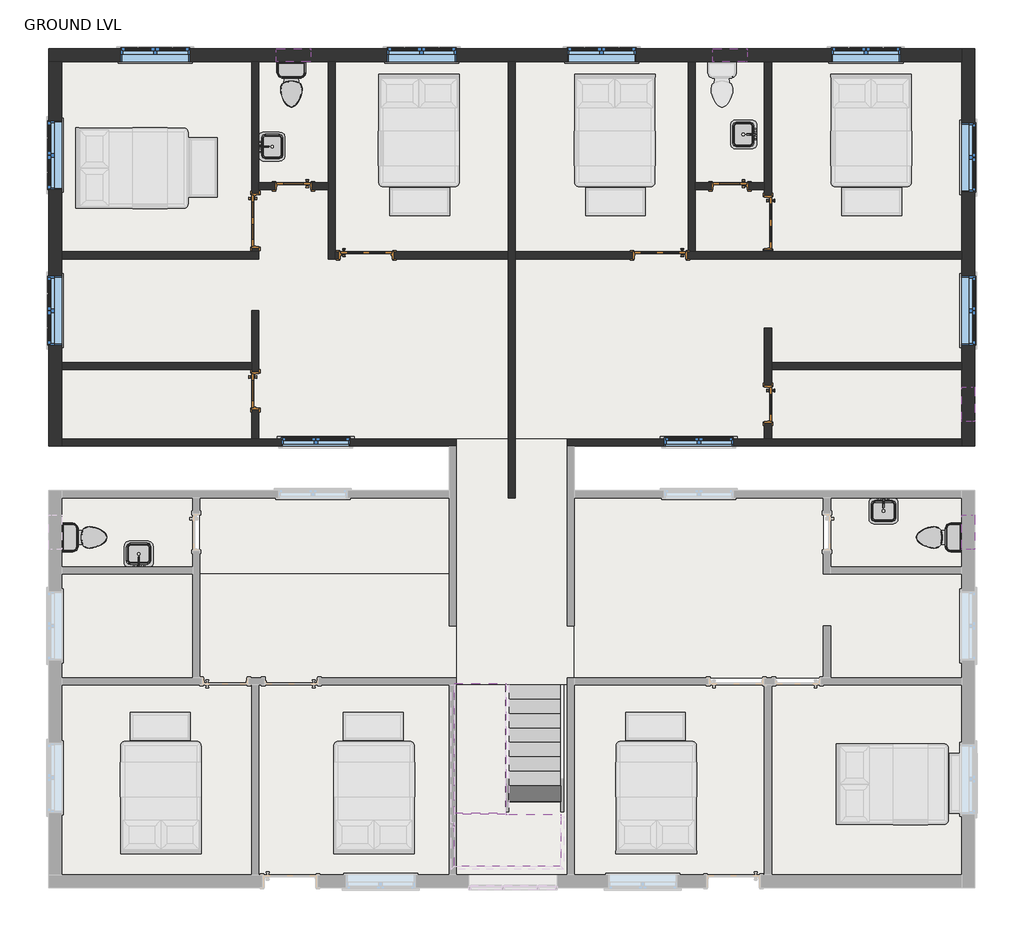
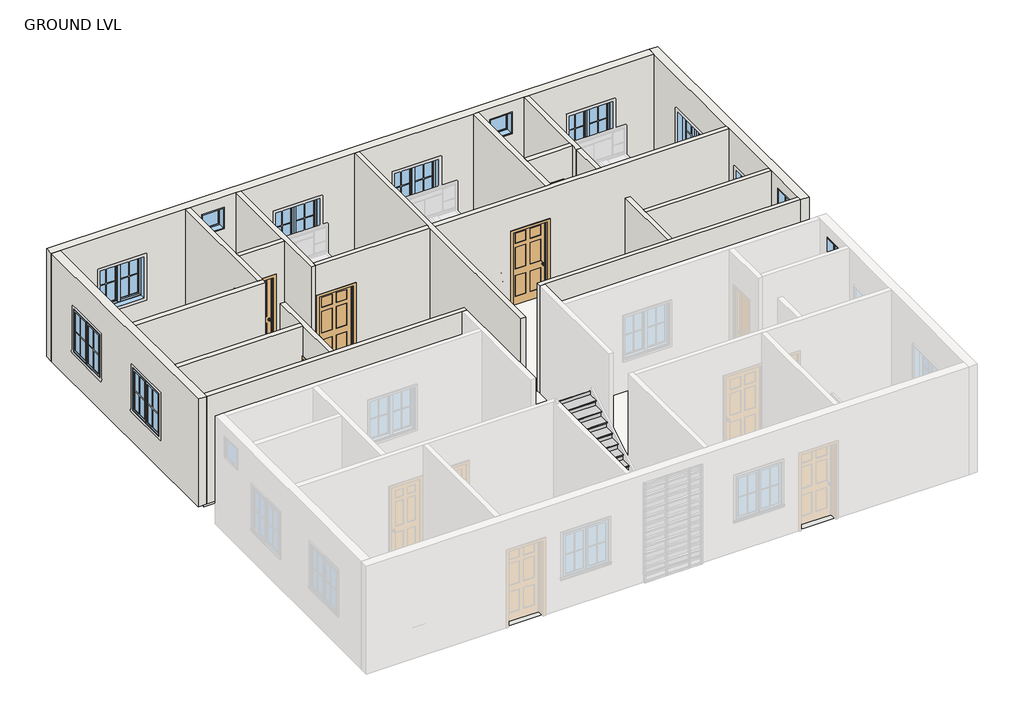
# One storey, part 3 of 4: 20 walls, 14 windows, 8 doors, 7 flow terminals, 7 slabs, 2 stair flights.
"""IFC4 building model written with IfcOpenShell, lengths in millimetres."""

from ifc_helpers import new_model, si_unit, frame, origin, origin_with_axes, place, context, project, spatial, polyline, outline, extrude, faceted_brep, transform, mapped, element, save
from components import door_e337afa5, door_596d7c92, door_c610b25b, door_03e3dfb5, flow_terminal_8d9ea526, toilet_domestic_3d_toilet_domestic_3d_ba6479b0, toilet_domestic_3d_toilet_domestic_3d_30431060, non_monolithic_landing_2d37ff17, stair_flight_38cd46e1, stair_flight_39a519ea, window_80340324, window_9200f5ac, window_c2c97eee

model = new_model("IFC4")

# Units and contexts
model_context = context("Model", 3, world=origin())
ifc_project = project(units=[si_unit("LENGTHUNIT", "METRE", prefix="MILLI")], contexts=[model_context])

# Site, building, storey
site = spatial("IfcSite", under=ifc_project)
building = spatial("IfcBuilding", under=site)
storey = spatial("IfcBuildingStorey", under=building, Name="GROUND LVL", Elevation=0.0)

# Doors
placement = place(None, origin())
door_shape = door_e337afa5(model_context)
element("IfcDoor", 1, ObjectType="Door-Interior-Single-2_Panel-Wood : 24\" x 84\"", at=placement, inside=storey, context=model_context, shape_type="MappedRepresentation", body=[
    mapped(door_shape, transform((-8112.4137331, 4563.2156164, 0.0), x_axis=(-1.0, 0.0, 0.0), y_axis=(0.0, -1.0, 0.0), z_axis=(0.0, 0.0, 1.0))),
])
element("IfcDoor", 2, ObjectType="Door-Interior-Single-2_Panel-Wood : 24\" x 84\"", at=placement, inside=storey, context=model_context, shape_type="MappedRepresentation", body=[
    mapped(door_shape, transform((-416.2137331, 4563.2156164, 0.0), x_axis=(-1.0, 0.0, 0.0), y_axis=(0.0, -1.0, 0.0), z_axis=(0.0, 0.0, 1.0))),
])
element("IfcDoor", 3, ObjectType="Door-Interior-Single-2_Panel-Wood : 24\" x 84\"", at=placement, inside=storey, context=model_context, shape_type="MappedRepresentation", body=[
    mapped(door_shape, transform((-8788.6887331, 953.2406164, 0.0), x_axis=(0.0, -1.0, 0.0), y_axis=(1.0, 0.0, 0.0), z_axis=(0.0, 0.0, 1.0))),
])
door_2_shape = door_596d7c92(model_context)
element("IfcDoor", 4, ObjectType="Door-Interior-Single-2_Panel-Wood : 24\" x 84\"", at=placement, inside=storey, context=model_context, shape_type="MappedRepresentation", body=[
    mapped(door_2_shape, transform((260.0612669, 711.9406164, 0.0), x_axis=(0.0, -1.0, 0.0), y_axis=(1.0, 0.0, 0.0), z_axis=(0.0, 0.0, 1.0))),
])
door_3_shape = door_c610b25b(model_context)
element("IfcDoor", 5, ObjectType="Door-Interior-Single-6_Panel-Wood : 36\" x 84\"", at=placement, inside=storey, context=model_context, shape_type="MappedRepresentation", body=[
    mapped(door_3_shape, transform((-8788.6887331, 3950.4406164, 0.0), x_axis=(0.0, -1.0, 0.0), y_axis=(1.0, 0.0, 0.0), z_axis=(0.0, 0.0, 1.0))),
])
element("IfcDoor", 6, ObjectType="Door-Interior-Single-6_Panel-Wood : 36\" x 84\"", at=placement, inside=storey, context=model_context, shape_type="MappedRepresentation", body=[
    mapped(door_3_shape, transform((-1648.1137331, 3344.0156164, 0.0), x_axis=(-1.0, 0.0, 0.0), y_axis=(0.0, -1.0, 0.0), z_axis=(0.0, 0.0, 1.0))),
])
door_4_shape = door_03e3dfb5(model_context)
element("IfcDoor", 7, ObjectType="Door-Interior-Single-6_Panel-Wood : 36\" x 84\"", at=placement, inside=storey, context=model_context, shape_type="MappedRepresentation", body=[
    mapped(door_4_shape, transform((-6829.7137331, 3344.0156164, 0.0), x_axis=(1.0, 0.0, 0.0), y_axis=(0.0, 1.0, 0.0), z_axis=(0.0, 0.0, 1.0))),
])
element("IfcDoor", 8, ObjectType="Door-Interior-Single-6_Panel-Wood : 36\" x 84\"", at=placement, inside=storey, context=model_context, shape_type="MappedRepresentation", body=[
    mapped(door_4_shape, transform((260.0612669, 3912.3406164, 0.0), x_axis=(0.0, -1.0, 0.0), y_axis=(1.0, 0.0, 0.0), z_axis=(0.0, 0.0, 1.0))),
])

# Flow terminals
flow_terminal_shape = flow_terminal_8d9ea526(model_context)
element("IfcFlowTerminal", 9, ObjectType="Sink Vanity-Square : 20\" x 18\"", at=placement, inside=storey, context=model_context, shape_type="MappedRepresentation", body=[
    mapped(flow_terminal_shape, transform((-8541.868332, 5244.4388758, 0.0), x_axis=(0.0, 1.0, 0.0), y_axis=(-1.0, 0.0, 0.0), z_axis=(0.0, 0.0, 1.0))),
])
element("IfcFlowTerminal", 10, ObjectType="Sink Vanity-Square : 20\" x 18\"", at=placement, inside=storey, context=model_context, shape_type="MappedRepresentation", body=[
    mapped(flow_terminal_shape, transform((-126.4240396, 5490.129857, 0.0), x_axis=(0.0, -1.0, 0.0), y_axis=(1.0, 0.0, 0.0), z_axis=(0.0, 0.0, 1.0))),
])
element("IfcFlowTerminal", 11, ObjectType="Sink Vanity-Square : 20\" x 18\"", at=placement, inside=storey, context=model_context, shape_type="MappedRepresentation", body=[
    mapped(flow_terminal_shape, transform((2277.6299024, -1119.2047847, 0.0), x_axis=(1.0, 0.0, 0.0), y_axis=(0.0, 1.0, 0.0), z_axis=(0.0, 0.0, 1.0))),
])
element("IfcFlowTerminal", 12, ObjectType="Sink Vanity-Square : 20\" x 18\"", at=placement, inside=storey, context=model_context, shape_type="MappedRepresentation", body=[
    mapped(flow_terminal_shape, transform((-10827.2244926, -1978.1139825, 0.0), x_axis=(-1.0, 0.0, 0.0), y_axis=(0.0, -1.0, 0.0), z_axis=(0.0, 0.0, 1.0))),
])
toilet_domestic_3d_toilet_domestic_3d_shape = toilet_domestic_3d_toilet_domestic_3d_ba6479b0(model_context)
toilet_domestic_3d_toilet_domestic_3d_2_shape = toilet_domestic_3d_toilet_domestic_3d_30431060(model_context)
element("IfcFlowTerminal", 13, ObjectType="Toilet-Domestic-3D : Toilet-Domestic-3D", at=placement, inside=storey, context=model_context, shape_type="MappedRepresentation", body=[
    mapped(toilet_domestic_3d_toilet_domestic_3d_shape, transform((-8150.5137331, 6264.032089, 0.0), x_axis=(1.0, 0.0, 0.0), y_axis=(0.0, 1.0, 0.0), z_axis=(0.0, 0.0, 1.0))),
    mapped(toilet_domestic_3d_toilet_domestic_3d_2_shape, transform((-8150.5137331, 6264.032089, 0.0), x_axis=(1.0, 0.0, 0.0), y_axis=(0.0, 1.0, 0.0), z_axis=(0.0, 0.0, 1.0))),
])
element("IfcFlowTerminal", 14, ObjectType="Toilet-Domestic-3D : Toilet-Domestic-3D", at=placement, inside=storey, context=model_context, shape_type="MappedRepresentation", body=[
    mapped(toilet_domestic_3d_toilet_domestic_3d_shape, transform((-11707.1177058, -1637.5593836, 0.0), x_axis=(0.0, 1.0, 0.0), y_axis=(-1.0, 0.0, 0.0), z_axis=(0.0, 0.0, 1.0))),
    mapped(toilet_domestic_3d_toilet_domestic_3d_2_shape, transform((-11707.1177058, -1637.5593836, 0.0), x_axis=(0.0, 1.0, 0.0), y_axis=(-1.0, 0.0, 0.0), z_axis=(0.0, 0.0, 1.0))),
])
element("IfcFlowTerminal", 15, ObjectType="Toilet-Domestic-3D : Toilet-Domestic-3D", at=placement, inside=storey, context=model_context, shape_type="MappedRepresentation", body=[
    mapped(toilet_domestic_3d_toilet_domestic_3d_shape, transform((3178.4902395, -1637.5593836, 0.0), x_axis=(0.0, -1.0, 0.0), y_axis=(1.0, 0.0, 0.0), z_axis=(0.0, 0.0, 1.0))),
    mapped(toilet_domestic_3d_toilet_domestic_3d_2_shape, transform((3178.4902395, -1637.5593836, 0.0), x_axis=(0.0, -1.0, 0.0), y_axis=(1.0, 0.0, 0.0), z_axis=(0.0, 0.0, 1.0))),
])

# Slabs
non_monolithic_landing_shape = non_monolithic_landing_2d37ff17(model_context)
element("IfcSlab", 16, ObjectType="Non-Monolithic Landing", at=placement, inside=storey, context=model_context, shape_type="MappedRepresentation", body=[
    mapped(non_monolithic_landing_shape, transform((0.0, 0.0, 0.0), x_axis=(1.0, 0.0, 0.0), y_axis=(0.0, 1.0, 0.0), z_axis=(0.0, 0.0, 1.0))),
])
element("IfcSlab", 17, ObjectType="marble tiles", at=placement, inside=storey, context=model_context, shape_type="SweptSolid", body=[
    extrude(outline(polyline([(-9890.4137331, -939.0593836), (-9890.4137331, -2158.2593836), (-12201.8137331, -2158.2593836), (-12201.8137331, -939.0593836), (-9890.4137331, -939.0593836)])), frame((0.0, 0.0, -152.4), z_axis=(0.0, 0.0, 1.0), x_axis=(1.0, 0.0, 0.0)), (0.0, 0.0, 1.0), 152.4),
    extrude(outline(polyline([(3673.1862669, -2158.2593836), (1361.7862669, -2158.2593836), (1361.7862669, -939.0593836), (3673.1862669, -939.0593836), (3673.1862669, -2158.2593836)])), frame((0.0, 0.0, -152.4), z_axis=(0.0, 0.0, 1.0), x_axis=(1.0, 0.0, 0.0)), (0.0, 0.0, 1.0), 152.4),
    extrude(outline(polyline([(-7502.8137331, 6758.7281164), (-7502.8137331, 4623.5406164), (-8722.0137331, 4623.5406164), (-8722.0137331, 6758.7281164), (-7502.8137331, 6758.7281164)])), frame((0.0, 0.0, -152.4), z_axis=(0.0, 0.0, 1.0), x_axis=(1.0, 0.0, 0.0)), (0.0, 0.0, 1.0), 152.4),
    extrude(outline(polyline([(193.3862669, 4623.5406164), (-1025.8137331, 4623.5406164), (-1025.8137331, 6758.7281164), (193.3862669, 6758.7281164), (193.3862669, 4623.5406164)])), frame((0.0, 0.0, -152.4), z_axis=(0.0, 0.0, 1.0), x_axis=(1.0, 0.0, 0.0)), (0.0, 0.0, 1.0), 152.4),
])
element("IfcSlab", 18, ObjectType="marble tiles", at=placement, inside=storey, context=model_context, shape_type="SweptSolid", body=[
    extrude(outline(polyline([(3673.1862669, 102.3406164), (-12201.8137331, 102.3406164), (-12201.8137331, 6758.7281164), (3673.1862669, 6758.7281164), (3673.1862669, 102.3406164)])), frame((0.0, 0.0, -152.4), z_axis=(0.0, 0.0, 1.0), x_axis=(1.0, 0.0, 0.0)), (0.0, 0.0, 1.0), 152.4),
])
element("IfcSlab", 19, ObjectType="marble tiles", at=placement, inside=storey, context=model_context, shape_type="SweptSolid", body=[
    extrude(outline(polyline([(-5242.2137331, -7593.8593836), (-12201.8137331, -7593.8593836), (-12201.8137331, -2285.2593836), (-5242.2137331, -2285.2593836), (-5242.2137331, -7593.8593836)])), frame((0.0, 0.0, -152.4), z_axis=(0.0, 0.0, 1.0), x_axis=(1.0, 0.0, 0.0)), (0.0, 0.0, 1.0), 152.4),
])
element("IfcSlab", 20, ObjectType="marble tiles", at=placement, inside=storey, context=model_context, shape_type="SweptSolid", body=[
    extrude(outline(polyline([(-5242.2137331, -2285.2593836), (-9763.4137331, -2285.2593836), (-9763.4137331, -812.0593836), (-5242.2137331, -812.0593836), (-5242.2137331, -2285.2593836)])), frame((0.0, 0.0, -152.4), z_axis=(0.0, 0.0, 1.0), x_axis=(1.0, 0.0, 0.0)), (0.0, 0.0, 1.0), 152.4),
])
element("IfcSlab", 21, ObjectType="marble tiles", at=placement, inside=storey, context=model_context, shape_type="SweptSolid", body=[
    extrude(outline(polyline([(-3159.4137331, -4241.0593836), (-5242.2137331, -4241.0593836), (-5242.2137331, 102.3406164), (-3159.4137331, 102.3406164), (-3159.4137331, -4241.0593836)])), frame((0.0, 0.0, -152.4), z_axis=(0.0, 0.0, 1.0), x_axis=(1.0, 0.0, 0.0)), (0.0, 0.0, 1.0), 152.4),
])
element("IfcSlab", 22, ObjectType="marble tiles", at=placement, inside=storey, context=model_context, shape_type="SweptSolid", body=[
    extrude(outline(polyline([(-3286.4137331, -7593.8593836), (-5242.2137331, -7593.8593836), (-5242.2137331, -4241.0593836), (-3286.4137331, -4241.0593836), (-3286.4137331, -7593.8593836)])), frame((0.0, 0.0, -152.4), z_axis=(0.0, 0.0, 1.0), x_axis=(1.0, 0.0, 0.0)), (0.0, 0.0, 1.0), 152.4),
    extrude(outline(polyline([(193.3862669, -7593.8593836), (-3159.4137331, -7593.8593836), (-3159.4137331, -4241.0593836), (193.3862669, -4241.0593836), (193.3862669, -7593.8593836)])), frame((0.0, 0.0, -152.4), z_axis=(0.0, 0.0, 1.0), x_axis=(1.0, 0.0, 0.0)), (0.0, 0.0, 1.0), 152.4),
    extrude(outline(polyline([(3673.1862669, -7593.8593836), (320.3862669, -7593.8593836), (320.3862669, -4241.0593836), (3673.1862669, -4241.0593836), (3673.1862669, -7593.8593836)])), frame((0.0, 0.0, -152.4), z_axis=(0.0, 0.0, 1.0), x_axis=(1.0, 0.0, 0.0)), (0.0, 0.0, 1.0), 152.4),
    extrude(outline(polyline([(1234.7862669, -4114.0593836), (-3159.4137331, -4114.0593836), (-3159.4137331, -939.0593836), (1234.7862669, -939.0593836), (1234.7862669, -2285.2593836), (3673.1862669, -2285.2593836), (3673.1862669, -4114.0593836), (1234.7862669, -4114.0593836)])), frame((0.0, 0.0, -152.4), z_axis=(0.0, 0.0, 1.0), x_axis=(1.0, 0.0, 0.0)), (0.0, 0.0, 1.0), 152.4),
])

# Stair flights
stair_flight_shape = stair_flight_38cd46e1(model_context)
element("IfcStairFlight", 23, ObjectType="2\" Tread 1\" Nosing 1/4\" Riser", at=placement, inside=storey, context=model_context, shape_type="MappedRepresentation", body=[
    mapped(stair_flight_shape, transform((0.0, 0.0, 0.0), x_axis=(1.0, 0.0, 0.0), y_axis=(0.0, 1.0, 0.0), z_axis=(0.0, 0.0, 1.0))),
])
stair_flight_2_shape = stair_flight_39a519ea(model_context)
element("IfcStairFlight", 24, ObjectType="2\" Tread 1\" Nosing 1/4\" Riser", at=placement, inside=storey, context=model_context, shape_type="MappedRepresentation", body=[
    mapped(stair_flight_2_shape, transform((0.0, 0.0, 0.0), x_axis=(1.0, 0.0, 0.0), y_axis=(0.0, 1.0, 0.0), z_axis=(0.0, 0.0, 1.0))),
])

# Walls
element("IfcWall", 25, ObjectType="Inner Wall 5\"", at=placement, inside=storey, context=model_context, shape_type="Brep", body=[
    faceted_brep([(-12201.8137331, -24.6593836, 0.0), (-5369.2137331, -24.6593836, 0.0), (-5242.2137331, -24.6593836, 0.0), (-5242.2137331, -24.6593836, 3048.0), (-5369.2137331, -24.6593836, 3048.0), (-12201.8137331, -24.6593836, 3048.0), (-7109.1137331, -24.6593836, 2133.6), (-7109.1137331, -24.6593836, 914.4), (-8328.3137331, -24.6593836, 914.4), (-8328.3137331, -24.6593836, 2133.6), (-12201.8137331, 102.3406164, 0.0), (-12201.8137331, 102.3406164, 3048.0), (-8849.0137331, 102.3406164, 3048.0), (-8722.0137331, 102.3406164, 3048.0), (-5242.2137331, 102.3406164, 3048.0), (-5242.2137331, 102.3406164, 0.0), (-8722.0137331, 102.3406164, 0.0), (-8849.0137331, 102.3406164, 0.0), (-7109.1137331, 102.3406164, 2133.6), (-8328.3137331, 102.3406164, 2133.6), (-8328.3137331, 102.3406164, 914.4), (-7109.1137331, 102.3406164, 914.4)], [[[0, 1, 2, 3, 4, 5], [6, 7, 8, 9]], [[10, 11, 12, 13, 14, 15, 16, 17], [18, 19, 20, 21]], [[2, 1, 0, 10, 17, 16, 15]], [[0, 5, 11, 10]], [[3, 2, 15, 14]], [[7, 6, 18, 21]], [[8, 7, 21, 20]], [[9, 8, 20, 19]], [[6, 9, 19, 18]], [[5, 4, 3, 14, 13, 12, 11]]]),
])
element("IfcWall", 26, ObjectType="Inner Wall 5\"", at=placement, inside=storey, context=model_context, shape_type="Brep", body=[
    faceted_brep([(3673.1862669, 102.3406164, 0.0), (320.3862669, 102.3406164, 0.0), (193.3862669, 102.3406164, 0.0), (-3286.4137331, 102.3406164, 0.0), (-3286.4137331, 102.3406164, 3048.0), (193.3862669, 102.3406164, 3048.0), (320.3862669, 102.3406164, 3048.0), (3673.1862669, 102.3406164, 3048.0), (-352.7137331, 102.3406164, 2133.6), (-1571.9137331, 102.3406164, 2133.6), (-1571.9137331, 102.3406164, 914.4), (-352.7137331, 102.3406164, 914.4), (3673.1862669, -24.6593836, 0.0), (3673.1862669, -24.6593836, 3048.0), (-3159.4137331, -24.6593836, 3048.0), (-3286.4137331, -24.6593836, 3048.0), (-3286.4137331, -24.6593836, 0.0), (-3159.4137331, -24.6593836, 0.0), (-352.7137331, -24.6593836, 2133.6), (-352.7137331, -24.6593836, 914.4), (-1571.9137331, -24.6593836, 914.4), (-1571.9137331, -24.6593836, 2133.6)], [[[0, 1, 2, 3, 4, 5, 6, 7], [8, 9, 10, 11]], [[12, 13, 14, 15, 16, 17], [18, 19, 20, 21]], [[3, 2, 1, 0, 12, 17, 16]], [[0, 7, 13, 12]], [[4, 3, 16, 15]], [[19, 18, 8, 11]], [[20, 19, 11, 10]], [[21, 20, 10, 9]], [[18, 21, 9, 8]], [[7, 6, 5, 4, 15, 14, 13]]]),
])
element("IfcWall", 27, ObjectType="Inner Wall 5\"", at=placement, inside=storey, context=model_context, shape_type="Brep", body=[
    faceted_brep([(-12201.8137331, 3277.3406164, 0.0), (-8722.0137331, 3277.3406164, 0.0), (-8722.0137331, 3277.3406164, 3048.0), (-12201.8137331, 3277.3406164, 3048.0), (-12201.8137331, 3404.3406164, 0.0), (-12201.8137331, 3404.3406164, 3048.0), (-8849.0137331, 3404.3406164, 3048.0), (-8722.0137331, 3404.3406164, 3048.0), (-8722.0137331, 3404.3406164, 0.0), (-8849.0137331, 3404.3406164, 0.0)], [[[0, 1, 2, 3]], [[4, 5, 6, 7, 8, 9]], [[1, 0, 4, 9, 8]], [[0, 3, 5, 4]], [[2, 1, 8, 7]], [[3, 2, 7, 6, 5]]]),
])
element("IfcWall", 28, ObjectType="Inner Wall 5\"", at=placement, inside=storey, context=model_context, shape_type="Brep", body=[
    faceted_brep([(-8722.0137331, 3404.3406164, 3048.0), (-8722.0137331, 3404.3406164, 0.0), (-8722.0137331, 3467.8406164, 0.0), (-8722.0137331, 3467.8406164, 2159.0), (-8722.0137331, 4433.0406164, 2159.0), (-8722.0137331, 4433.0406164, 0.0), (-8722.0137331, 4496.5406164, 0.0), (-8722.0137331, 4623.5406164, 0.0), (-8722.0137331, 6758.7281164, 0.0), (-8722.0137331, 6758.7281164, 3048.0), (-8722.0137331, 4623.5406164, 3048.0), (-8722.0137331, 4496.5406164, 3048.0), (-8849.0137331, 3404.3406164, 0.0), (-8849.0137331, 3404.3406164, 3048.0), (-8849.0137331, 6758.7281164, 3048.0), (-8849.0137331, 6758.7281164, 0.0), (-8849.0137331, 4433.0406164, 0.0), (-8849.0137331, 4433.0406164, 2159.0), (-8849.0137331, 3467.8406164, 2159.0), (-8849.0137331, 3467.8406164, 0.0)], [[[0, 1, 2, 3, 4, 5, 6, 7, 8, 9, 10, 11]], [[12, 13, 14, 15, 16, 17, 18, 19]], [[1, 12, 19, 2]], [[15, 8, 7, 6, 5, 16]], [[1, 0, 13, 12]], [[9, 8, 15, 14]], [[18, 3, 2, 19]], [[3, 18, 17, 4]], [[4, 17, 16, 5]], [[0, 11, 10, 9, 14, 13]]]),
])
element("IfcWall", 29, ObjectType="Inner Wall 5\"", at=placement, inside=storey, context=model_context, shape_type="SweptSolid", body=[
    extrude(outline(polyline([(3048.0, -8722.0137331), (0.0, -8722.0137331), (0.0, -8442.6137331), (2159.0, -8442.6137331), (2159.0, -7782.2137331), (0.0, -7782.2137331), (0.0, -7502.8137331), (3048.0, -7502.8137331), (3048.0, -8722.0137331)])), frame((0.0, 4496.5406164, 0.0), z_axis=(0.0, 1.0, 0.0), x_axis=(0.0, 0.0, 1.0)), (0.0, 0.0, 1.0), 127.0),
])
element("IfcWall", 30, ObjectType="Inner Wall 5\"", at=placement, inside=storey, context=model_context, shape_type="Brep", body=[
    faceted_brep([(-7375.8137331, 3277.3406164, 0.0), (-7375.8137331, 3404.3406164, 0.0), (-7375.8137331, 6758.7281164, 0.0), (-7375.8137331, 6758.7281164, 3048.0), (-7375.8137331, 3404.3406164, 3048.0), (-7375.8137331, 3277.3406164, 3048.0), (-7502.8137331, 3277.3406164, 0.0), (-7502.8137331, 3277.3406164, 3048.0), (-7502.8137331, 4496.5406164, 3048.0), (-7502.8137331, 4623.5406164, 3048.0), (-7502.8137331, 6758.7281164, 3048.0), (-7502.8137331, 6758.7281164, 0.0), (-7502.8137331, 4623.5406164, 0.0), (-7502.8137331, 4496.5406164, 0.0)], [[[0, 1, 2, 3, 4, 5]], [[6, 7, 8, 9, 10, 11, 12, 13]], [[2, 1, 0, 6, 13, 12, 11]], [[3, 2, 11, 10]], [[0, 5, 7, 6]], [[5, 4, 3, 10, 9, 8, 7]]]),
])
element("IfcWall", 31, ObjectType="Inner Wall 5\"", at=placement, inside=storey, context=model_context, shape_type="Brep", body=[
    faceted_brep([(-4327.8137331, 6758.7281164, 0.0), (-4327.8137331, 3404.3406164, 0.0), (-4327.8137331, 3277.3406164, 0.0), (-4327.8137331, -939.0593836, 0.0), (-4327.8137331, -939.0593836, 3048.0), (-4327.8137331, 3277.3406164, 3048.0), (-4327.8137331, 3404.3406164, 3048.0), (-4327.8137331, 6758.7281164, 3048.0), (-4200.8137331, 6758.7281164, 0.0), (-4200.8137331, 6758.7281164, 3048.0), (-4200.8137331, 3404.3406164, 3048.0), (-4200.8137331, 3277.3406164, 3048.0), (-4200.8137331, -939.0593836, 3048.0), (-4200.8137331, -939.0593836, 0.0), (-4200.8137331, 3277.3406164, 0.0), (-4200.8137331, 3404.3406164, 0.0)], [[[0, 1, 2, 3, 4, 5, 6, 7]], [[8, 9, 10, 11, 12, 13, 14, 15]], [[3, 2, 1, 0, 8, 15, 14, 13]], [[4, 3, 13, 12]], [[0, 7, 9, 8]], [[7, 6, 5, 4, 12, 11, 10, 9]]]),
])
element("IfcWall", 32, ObjectType="Inner Wall 5\"", at=placement, inside=storey, context=model_context, shape_type="SweptSolid", body=[
    extrude(outline(polyline([(3048.0, -7375.8137331), (0.0, -7375.8137331), (0.0, -7312.3137331), (2159.0, -7312.3137331), (2159.0, -6347.1137331), (0.0, -6347.1137331), (0.0, -4327.8137331), (3048.0, -4327.8137331), (3048.0, -7375.8137331)])), frame((0.0, 3277.3406164, 0.0), z_axis=(0.0, 1.0, 0.0), x_axis=(0.0, 0.0, 1.0)), (0.0, 0.0, 1.0), 127.0),
])
element("IfcWall", 33, ObjectType="Inner Wall 5\"", at=placement, inside=storey, context=model_context, shape_type="Brep", body=[
    faceted_brep([(-4200.8137331, 3277.3406164, 3048.0), (-4200.8137331, 3277.3406164, 0.0), (-2130.7137331, 3277.3406164, 0.0), (-2130.7137331, 3277.3406164, 2159.0), (-1165.5137331, 3277.3406164, 2159.0), (-1165.5137331, 3277.3406164, 0.0), (3673.1862669, 3277.3406164, 0.0), (3673.1862669, 3277.3406164, 3048.0), (-4200.8137331, 3404.3406164, 0.0), (-4200.8137331, 3404.3406164, 3048.0), (-1152.8137331, 3404.3406164, 3048.0), (-1025.8137331, 3404.3406164, 3048.0), (193.3862669, 3404.3406164, 3048.0), (320.3862669, 3404.3406164, 3048.0), (3673.1862669, 3404.3406164, 3048.0), (3673.1862669, 3404.3406164, 0.0), (320.3862669, 3404.3406164, 0.0), (193.3862669, 3404.3406164, 0.0), (-1025.8137331, 3404.3406164, 0.0), (-1152.8137331, 3404.3406164, 0.0), (-1165.5137331, 3404.3406164, 0.0), (-1165.5137331, 3404.3406164, 2159.0), (-2130.7137331, 3404.3406164, 2159.0), (-2130.7137331, 3404.3406164, 0.0)], [[[0, 1, 2, 3, 4, 5, 6, 7]], [[8, 9, 10, 11, 12, 13, 14, 15, 16, 17, 18, 19, 20, 21, 22, 23]], [[1, 8, 23, 2]], [[15, 6, 5, 20, 19, 18, 17, 16]], [[1, 0, 9, 8]], [[7, 6, 15, 14]], [[22, 3, 2, 23]], [[3, 22, 21, 4]], [[4, 21, 20, 5]], [[0, 7, 14, 13, 12, 11, 10, 9]]]),
])
element("IfcWall", 34, ObjectType="Inner Wall 5\"", at=placement, inside=storey, context=model_context, shape_type="Brep", body=[
    faceted_brep([(-1025.8137331, 3404.3406164, 0.0), (-1025.8137331, 4496.5406164, 0.0), (-1025.8137331, 4623.5406164, 0.0), (-1025.8137331, 6758.7281164, 0.0), (-1025.8137331, 6758.7281164, 3048.0), (-1025.8137331, 4623.5406164, 3048.0), (-1025.8137331, 4496.5406164, 3048.0), (-1025.8137331, 3404.3406164, 3048.0), (-1152.8137331, 3404.3406164, 0.0), (-1152.8137331, 3404.3406164, 3048.0), (-1152.8137331, 6758.7281164, 3048.0), (-1152.8137331, 6758.7281164, 0.0)], [[[0, 1, 2, 3, 4, 5, 6, 7]], [[8, 9, 10, 11]], [[3, 2, 1, 0, 8, 11]], [[0, 7, 9, 8]], [[4, 3, 11, 10]], [[7, 6, 5, 4, 10, 9]]]),
])
element("IfcWall", 35, ObjectType="Inner Wall 5\"", at=placement, inside=storey, context=model_context, shape_type="SweptSolid", body=[
    extrude(outline(polyline([(3048.0, -1025.8137331), (0.0, -1025.8137331), (0.0, -746.4137331), (2159.0, -746.4137331), (2159.0, -86.0137331), (0.0, -86.0137331), (0.0, 193.3862669), (3048.0, 193.3862669), (3048.0, -1025.8137331)])), frame((0.0, 4496.5406164, 0.0), z_axis=(0.0, 1.0, 0.0), x_axis=(0.0, 0.0, 1.0)), (0.0, 0.0, 1.0), 127.0),
])
element("IfcWall", 36, ObjectType="Inner Wall 5\"", at=placement, inside=storey, context=model_context, shape_type="Brep", body=[
    faceted_brep([(320.3862669, 6758.7281164, 0.0), (320.3862669, 6758.7281164, 3048.0), (320.3862669, 4318.7406164, 3048.0), (320.3862669, 4318.7406164, 2159.0), (320.3862669, 4394.9406164, 2159.0), (320.3862669, 4394.9406164, 0.0), (193.3862669, 6758.7281164, 3048.0), (193.3862669, 6758.7281164, 0.0), (193.3862669, 4623.5406164, 0.0), (193.3862669, 4496.5406164, 0.0), (193.3862669, 4394.9406164, 0.0), (193.3862669, 4394.9406164, 2159.0), (193.3862669, 4318.7406164, 2159.0), (193.3862669, 4318.7406164, 3048.0), (193.3862669, 4496.5406164, 3048.0), (193.3862669, 4623.5406164, 3048.0)], [[[0, 1, 2, 3, 4, 5]], [[6, 7, 8, 9, 10, 11, 12, 13, 14, 15]], [[7, 0, 5, 10, 9, 8]], [[2, 13, 12, 3]], [[1, 0, 7, 6]], [[11, 4, 3, 12]], [[4, 11, 10, 5]], [[2, 1, 6, 15, 14, 13]]]),
])
element("IfcWall", 37, ObjectType="Inner Wall 5\"", at=placement, inside=storey, context=model_context, shape_type="SweptSolid", body=[
    extrude(outline(polyline([(320.3862669, 1448.5406164), (3673.1862669, 1448.5406164), (3673.1862669, 1321.5406164), (320.3862669, 1321.5406164), (320.3862669, 1448.5406164)])), origin_with_axes(), (0.0, 0.0, 1.0), 3048.0),
])
element("IfcWall", 38, ObjectType="Inner Wall 5\"", at=placement, inside=storey, context=model_context, shape_type="Brep", body=[
    faceted_brep([(193.3862669, 2058.1406164, 3048.0), (193.3862669, 2058.1406164, 0.0), (193.3862669, 1042.1406164, 0.0), (193.3862669, 1042.1406164, 2159.0), (193.3862669, 381.7406164, 2159.0), (193.3862669, 381.7406164, 0.0), (193.3862669, 102.3406164, 0.0), (193.3862669, 102.3406164, 3048.0), (320.3862669, 2058.1406164, 0.0), (320.3862669, 2058.1406164, 3048.0), (320.3862669, 1448.5406164, 3048.0), (320.3862669, 1321.5406164, 3048.0), (320.3862669, 102.3406164, 3048.0), (320.3862669, 102.3406164, 0.0), (320.3862669, 381.7406164, 0.0), (320.3862669, 381.7406164, 2159.0), (320.3862669, 1042.1406164, 2159.0), (320.3862669, 1042.1406164, 0.0), (320.3862669, 1321.5406164, 0.0), (320.3862669, 1448.5406164, 0.0)], [[[0, 1, 2, 3, 4, 5, 6, 7]], [[8, 9, 10, 11, 12, 13, 14, 15, 16, 17, 18, 19]], [[1, 8, 19, 18, 17, 2]], [[13, 6, 5, 14]], [[1, 0, 9, 8]], [[7, 6, 13, 12]], [[4, 15, 14, 5]], [[15, 4, 3, 16]], [[16, 3, 2, 17]], [[0, 7, 12, 11, 10, 9]]]),
])
element("IfcWall", 39, ObjectType="Inner Wall 5\"", at=placement, inside=storey, context=model_context, shape_type="Brep", body=[
    faceted_brep([(-8722.0137331, 2362.9406164, 0.0), (-8722.0137331, 2362.9406164, 3048.0), (-8722.0137331, 102.3406164, 3048.0), (-8722.0137331, 102.3406164, 0.0), (-8722.0137331, 623.0406164, 0.0), (-8722.0137331, 623.0406164, 2159.0), (-8722.0137331, 1283.4406164, 2159.0), (-8722.0137331, 1283.4406164, 0.0), (-8849.0137331, 2362.9406164, 3048.0), (-8849.0137331, 2362.9406164, 0.0), (-8849.0137331, 1448.5406164, 0.0), (-8849.0137331, 1321.5406164, 0.0), (-8849.0137331, 1283.4406164, 0.0), (-8849.0137331, 1283.4406164, 2159.0), (-8849.0137331, 623.0406164, 2159.0), (-8849.0137331, 623.0406164, 0.0), (-8849.0137331, 102.3406164, 0.0), (-8849.0137331, 102.3406164, 3048.0), (-8849.0137331, 1321.5406164, 3048.0), (-8849.0137331, 1448.5406164, 3048.0)], [[[0, 1, 2, 3, 4, 5, 6, 7]], [[8, 9, 10, 11, 12, 13, 14, 15, 16, 17, 18, 19]], [[9, 0, 7, 12, 11, 10]], [[3, 16, 15, 4]], [[1, 0, 9, 8]], [[3, 2, 17, 16]], [[14, 5, 4, 15]], [[5, 14, 13, 6]], [[6, 13, 12, 7]], [[2, 1, 8, 19, 18, 17]]]),
])
element("IfcWall", 40, ObjectType="Inner Wall 5\"", at=placement, inside=storey, context=model_context, shape_type="SweptSolid", body=[
    extrude(outline(polyline([(-12201.8137331, 1448.5406164), (-8849.0137331, 1448.5406164), (-8849.0137331, 1321.5406164), (-12201.8137331, 1321.5406164), (-12201.8137331, 1448.5406164)])), origin_with_axes(), (0.0, 0.0, 1.0), 3048.0),
])
element("IfcWall", 41, ObjectType="Inner Wall 5\"", at=placement, inside=storey, context=model_context, shape_type="SweptSolid", body=[
    extrude(outline(polyline([(3404.3406164, 0.0), (3404.3406164, 3048.0), (4318.7406164, 3048.0), (4318.7406164, 2159.0), (3429.7406164, 2159.0), (3429.7406164, 0.0), (3404.3406164, 0.0)])), frame((193.3862669, 0.0, 0.0), z_axis=(1.0, 0.0, 0.0), x_axis=(0.0, 1.0, 0.0)), (0.0, 0.0, 1.0), 127.0),
])
element("IfcWall", 42, ObjectType="outer wall 9\"", at=placement, inside=storey, context=model_context, shape_type="Brep", body=[
    faceted_brep([(-12430.4137331, 6758.7281164, 0.0), (-12201.8137331, 6758.7281164, 0.0), (-8849.0137331, 6758.7281164, 0.0), (-8722.0137331, 6758.7281164, 0.0), (-7502.8137331, 6758.7281164, 0.0), (-7375.8137331, 6758.7281164, 0.0), (-4327.8137331, 6758.7281164, 0.0), (-4200.8137331, 6758.7281164, 0.0), (-1152.8137331, 6758.7281164, 0.0), (-1025.8137331, 6758.7281164, 0.0), (193.3862669, 6758.7281164, 0.0), (320.3862669, 6758.7281164, 0.0), (3673.1862669, 6758.7281164, 0.0), (3673.1862669, 6758.7281164, 3048.0), (320.3862669, 6758.7281164, 3048.0), (193.3862669, 6758.7281164, 3048.0), (-1025.8137331, 6758.7281164, 3048.0), (-1152.8137331, 6758.7281164, 3048.0), (-4200.8137331, 6758.7281164, 3048.0), (-4327.8137331, 6758.7281164, 3048.0), (-7375.8137331, 6758.7281164, 3048.0), (-7502.8137331, 6758.7281164, 3048.0), (-8722.0137331, 6758.7281164, 3048.0), (-8849.0137331, 6758.7281164, 3048.0), (-12201.8137331, 6758.7281164, 3048.0), (-12430.4137331, 6758.7281164, 3048.0), (-9941.2137331, 6758.7281164, 2133.6), (-9941.2137331, 6758.7281164, 914.4), (-11160.4137331, 6758.7281164, 914.4), (-11160.4137331, 6758.7281164, 2133.6), (-5242.2137331, 6758.7281164, 2133.6), (-5242.2137331, 6758.7281164, 914.4), (-6461.4137331, 6758.7281164, 914.4), (-6461.4137331, 6758.7281164, 2133.6), (-2067.2137331, 6758.7281164, 2133.6), (-2067.2137331, 6758.7281164, 914.4), (-3286.4137331, 6758.7281164, 914.4), (-3286.4137331, 6758.7281164, 2133.6), (2593.6862669, 6758.7281164, 2133.6), (2593.6862669, 6758.7281164, 914.4), (1374.4862669, 6758.7281164, 914.4), (1374.4862669, 6758.7281164, 2133.6), (-7807.6137331, 6758.7281164, 2743.2), (-7807.6137331, 6758.7281164, 2133.6), (-8417.2137331, 6758.7281164, 2133.6), (-8417.2137331, 6758.7281164, 2743.2), (-111.4137331, 6758.7281164, 2743.2), (-111.4137331, 6758.7281164, 2133.6), (-721.0137331, 6758.7281164, 2133.6), (-721.0137331, 6758.7281164, 2743.2), (-12430.4137331, 6987.3281164, 0.0), (-12430.4137331, 6987.3281164, 3048.0), (3673.1862669, 6987.3281164, 3048.0), (3673.1862669, 6987.3281164, 0.0), (-9941.2137331, 6987.3281164, 2133.6), (-11160.4137331, 6987.3281164, 2133.6), (-11160.4137331, 6987.3281164, 914.4), (-9941.2137331, 6987.3281164, 914.4), (-5242.2137331, 6987.3281164, 2133.6), (-6461.4137331, 6987.3281164, 2133.6), (-6461.4137331, 6987.3281164, 914.4), (-5242.2137331, 6987.3281164, 914.4), (-2067.2137331, 6987.3281164, 2133.6), (-3286.4137331, 6987.3281164, 2133.6), (-3286.4137331, 6987.3281164, 914.4), (-2067.2137331, 6987.3281164, 914.4), (2593.6862669, 6987.3281164, 2133.6), (1374.4862669, 6987.3281164, 2133.6), (1374.4862669, 6987.3281164, 914.4), (2593.6862669, 6987.3281164, 914.4), (-7807.6137331, 6987.3281164, 2743.2), (-8417.2137331, 6987.3281164, 2743.2), (-8417.2137331, 6987.3281164, 2133.6), (-7807.6137331, 6987.3281164, 2133.6), (-111.4137331, 6987.3281164, 2743.2), (-721.0137331, 6987.3281164, 2743.2), (-721.0137331, 6987.3281164, 2133.6), (-111.4137331, 6987.3281164, 2133.6)], [[[0, 1, 2, 3, 4, 5, 6, 7, 8, 9, 10, 11, 12, 13, 14, 15, 16, 17, 18, 19, 20, 21, 22, 23, 24, 25], [26, 27, 28, 29], [30, 31, 32, 33], [34, 35, 36, 37], [38, 39, 40, 41], [42, 43, 44, 45], [46, 47, 48, 49]], [[50, 51, 52, 53], [54, 55, 56, 57], [58, 59, 60, 61], [62, 63, 64, 65], [66, 67, 68, 69], [70, 71, 72, 73], [74, 75, 76, 77]], [[12, 11, 10, 9, 8, 7, 6, 5, 4, 3, 2, 1, 0, 50, 53]], [[0, 25, 51, 50]], [[13, 12, 53, 52]], [[27, 26, 54, 57]], [[28, 27, 57, 56]], [[29, 28, 56, 55]], [[26, 29, 55, 54]], [[31, 30, 58, 61]], [[32, 31, 61, 60]], [[33, 32, 60, 59]], [[30, 33, 59, 58]], [[35, 34, 62, 65]], [[36, 35, 65, 64]], [[37, 36, 64, 63]], [[34, 37, 63, 62]], [[39, 38, 66, 69]], [[40, 39, 69, 68]], [[41, 40, 68, 67]], [[38, 41, 67, 66]], [[43, 42, 70, 73]], [[44, 43, 73, 72]], [[45, 44, 72, 71]], [[42, 45, 71, 70]], [[47, 46, 74, 77]], [[48, 47, 77, 76]], [[49, 48, 76, 75]], [[46, 49, 75, 74]], [[25, 24, 23, 22, 21, 20, 19, 18, 17, 16, 15, 14, 13, 52, 51]]]),
])
element("IfcWall", 43, ObjectType="outer wall 9\"", at=placement, inside=storey, context=model_context, shape_type="Brep", body=[
    faceted_brep([(-12201.8137331, -24.6593836, 0.0), (-12201.8137331, 102.3406164, 0.0), (-12201.8137331, 1321.5406164, 0.0), (-12201.8137331, 1448.5406164, 0.0), (-12201.8137331, 3277.3406164, 0.0), (-12201.8137331, 3404.3406164, 0.0), (-12201.8137331, 6758.7281164, 0.0), (-12201.8137331, 6758.7281164, 3048.0), (-12201.8137331, 3404.3406164, 3048.0), (-12201.8137331, 3277.3406164, 3048.0), (-12201.8137331, 1448.5406164, 3048.0), (-12201.8137331, 1321.5406164, 3048.0), (-12201.8137331, 102.3406164, 3048.0), (-12201.8137331, -24.6593836, 3048.0), (-12201.8137331, 2972.5406164, 2133.6), (-12201.8137331, 2972.5406164, 914.4), (-12201.8137331, 1753.3406164, 914.4), (-12201.8137331, 1753.3406164, 2133.6), (-12201.8137331, 5716.5343664, 2133.6), (-12201.8137331, 5716.5343664, 914.4), (-12201.8137331, 4497.3343664, 914.4), (-12201.8137331, 4497.3343664, 2133.6), (-12430.4137331, -24.6593836, 0.0), (-12430.4137331, -24.6593836, 3048.0), (-12430.4137331, 6758.7281164, 3048.0), (-12430.4137331, 6758.7281164, 0.0), (-12430.4137331, 2972.5406164, 2133.6), (-12430.4137331, 1753.3406164, 2133.6), (-12430.4137331, 1753.3406164, 914.4), (-12430.4137331, 2972.5406164, 914.4), (-12430.4137331, 5716.5343664, 2133.6), (-12430.4137331, 4497.3343664, 2133.6), (-12430.4137331, 4497.3343664, 914.4), (-12430.4137331, 5716.5343664, 914.4)], [[[0, 1, 2, 3, 4, 5, 6, 7, 8, 9, 10, 11, 12, 13], [14, 15, 16, 17], [18, 19, 20, 21]], [[22, 23, 24, 25], [26, 27, 28, 29], [30, 31, 32, 33]], [[6, 5, 4, 3, 2, 1, 0, 22, 25]], [[7, 6, 25, 24]], [[0, 13, 23, 22]], [[15, 14, 26, 29]], [[16, 15, 29, 28]], [[17, 16, 28, 27]], [[14, 17, 27, 26]], [[19, 18, 30, 33]], [[20, 19, 33, 32]], [[21, 20, 32, 31]], [[18, 21, 31, 30]], [[13, 12, 11, 10, 9, 8, 7, 24, 23]]]),
])
element("IfcWall", 44, ObjectType="outer wall 9\"", at=placement, inside=storey, context=model_context, shape_type="Brep", body=[
    faceted_brep([(3673.1862669, 6987.3281164, 0.0), (3673.1862669, 6758.7281164, 0.0), (3673.1862669, 3404.3406164, 0.0), (3673.1862669, 3277.3406164, 0.0), (3673.1862669, 1448.5406164, 0.0), (3673.1862669, 1321.5406164, 0.0), (3673.1862669, 102.3406164, 0.0), (3673.1862669, -24.6593836, 0.0), (3673.1862669, -24.6593836, 3048.0), (3673.1862669, 102.3406164, 3048.0), (3673.1862669, 1321.5406164, 3048.0), (3673.1862669, 1448.5406164, 3048.0), (3673.1862669, 3277.3406164, 3048.0), (3673.1862669, 3404.3406164, 3048.0), (3673.1862669, 6758.7281164, 3048.0), (3673.1862669, 6987.3281164, 3048.0), (3673.1862669, 4458.4406164, 2133.6), (3673.1862669, 4458.4406164, 914.4), (3673.1862669, 5677.6406164, 914.4), (3673.1862669, 5677.6406164, 2133.6), (3673.1862669, 1753.3406164, 2133.6), (3673.1862669, 1753.3406164, 914.4), (3673.1862669, 2972.5406164, 914.4), (3673.1862669, 2972.5406164, 2133.6), (3673.1862669, 407.1406164, 2743.2), (3673.1862669, 407.1406164, 2133.6), (3673.1862669, 1016.7406164, 2133.6), (3673.1862669, 1016.7406164, 2743.2), (3901.7862669, 6987.3281164, 0.0), (3901.7862669, 6987.3281164, 3048.0), (3901.7862669, -24.6593836, 3048.0), (3901.7862669, -24.6593836, 0.0), (3901.7862669, 4458.4406164, 2133.6), (3901.7862669, 5677.6406164, 2133.6), (3901.7862669, 5677.6406164, 914.4), (3901.7862669, 4458.4406164, 914.4), (3901.7862669, 1753.3406164, 2133.6), (3901.7862669, 2972.5406164, 2133.6), (3901.7862669, 2972.5406164, 914.4), (3901.7862669, 1753.3406164, 914.4), (3901.7862669, 407.1406164, 2743.2), (3901.7862669, 1016.7406164, 2743.2), (3901.7862669, 1016.7406164, 2133.6), (3901.7862669, 407.1406164, 2133.6)], [[[0, 1, 2, 3, 4, 5, 6, 7, 8, 9, 10, 11, 12, 13, 14, 15], [16, 17, 18, 19], [20, 21, 22, 23], [24, 25, 26, 27]], [[28, 29, 30, 31], [32, 33, 34, 35], [36, 37, 38, 39], [40, 41, 42, 43]], [[7, 6, 5, 4, 3, 2, 1, 0, 28, 31]], [[0, 15, 29, 28]], [[8, 7, 31, 30]], [[17, 16, 32, 35]], [[18, 17, 35, 34]], [[19, 18, 34, 33]], [[16, 19, 33, 32]], [[21, 20, 36, 39]], [[22, 21, 39, 38]], [[23, 22, 38, 37]], [[20, 23, 37, 36]], [[25, 24, 40, 43]], [[26, 25, 43, 42]], [[27, 26, 42, 41]], [[24, 27, 41, 40]], [[15, 14, 13, 12, 11, 10, 9, 8, 30, 29]]]),
])

# Windows
window_shape = window_80340324(model_context)
element("IfcWindow", 45, ObjectType="Fixed : 24\" x 24\"", at=placement, inside=storey, context=model_context, shape_type="MappedRepresentation", body=[
    mapped(window_shape, transform((3787.4862669, -1586.7593836, 1219.2), x_axis=(0.0, -1.0, 0.0), y_axis=(1.0, 0.0, 0.0), z_axis=(0.0, 0.0, 1.0))),
])
element("IfcWindow", 46, ObjectType="Fixed : 24\" x 24\"", at=placement, inside=storey, context=model_context, shape_type="MappedRepresentation", body=[
    mapped(window_shape, transform((3787.4862669, 673.8406164, 1219.2), x_axis=(0.0, -1.0, 0.0), y_axis=(1.0, 0.0, 0.0), z_axis=(0.0, 0.0, 1.0))),
])
element("IfcWindow", 47, ObjectType="Fixed : 24\" x 24\"", at=placement, inside=storey, context=model_context, shape_type="MappedRepresentation", body=[
    mapped(window_shape, transform((-8074.3137331, 6873.0281164, 1219.2), x_axis=(1.0, 0.0, 0.0), y_axis=(0.0, 1.0, 0.0), z_axis=(0.0, 0.0, 1.0))),
])
element("IfcWindow", 48, ObjectType="Fixed : 24\" x 24\"", at=placement, inside=storey, context=model_context, shape_type="MappedRepresentation", body=[
    mapped(window_shape, transform((-378.1137331, 6873.0281164, 1219.2), x_axis=(1.0, 0.0, 0.0), y_axis=(0.0, 1.0, 0.0), z_axis=(0.0, 0.0, 1.0))),
])
window_2_shape = window_9200f5ac(model_context)
element("IfcWindow", 49, ObjectType="Window-Casement-Double : 48\" x 48\"", at=placement, inside=storey, context=model_context, shape_type="MappedRepresentation", body=[
    mapped(window_2_shape, transform((-12316.1137331, 2362.9406164, 0.0), x_axis=(0.0, 1.0, 0.0), y_axis=(-1.0, 0.0, 0.0), z_axis=(0.0, 0.0, 1.0))),
])
element("IfcWindow", 50, ObjectType="Window-Casement-Double : 48\" x 48\"", at=placement, inside=storey, context=model_context, shape_type="MappedRepresentation", body=[
    mapped(window_2_shape, transform((-12316.1137331, 5106.9343664, 0.0), x_axis=(0.0, 1.0, 0.0), y_axis=(-1.0, 0.0, 0.0), z_axis=(0.0, 0.0, 1.0))),
])
element("IfcWindow", 51, ObjectType="Window-Casement-Double : 48\" x 48\"", at=placement, inside=storey, context=model_context, shape_type="MappedRepresentation", body=[
    mapped(window_2_shape, transform((-10550.8137331, 6873.0281164, 0.0), x_axis=(1.0, 0.0, 0.0), y_axis=(0.0, 1.0, 0.0), z_axis=(0.0, 0.0, 1.0))),
])
element("IfcWindow", 52, ObjectType="Window-Casement-Double : 48\" x 48\"", at=placement, inside=storey, context=model_context, shape_type="MappedRepresentation", body=[
    mapped(window_2_shape, transform((-5851.8137331, 6873.0281164, 0.0), x_axis=(1.0, 0.0, 0.0), y_axis=(0.0, 1.0, 0.0), z_axis=(0.0, 0.0, 1.0))),
])
element("IfcWindow", 53, ObjectType="Window-Casement-Double : 48\" x 48\"", at=placement, inside=storey, context=model_context, shape_type="MappedRepresentation", body=[
    mapped(window_2_shape, transform((-2676.8137331, 6873.0281164, 0.0), x_axis=(1.0, 0.0, 0.0), y_axis=(0.0, 1.0, 0.0), z_axis=(0.0, 0.0, 1.0))),
])
element("IfcWindow", 54, ObjectType="Window-Casement-Double : 48\" x 48\"", at=placement, inside=storey, context=model_context, shape_type="MappedRepresentation", body=[
    mapped(window_2_shape, transform((1984.0862669, 6873.0281164, 0.0), x_axis=(1.0, 0.0, 0.0), y_axis=(0.0, 1.0, 0.0), z_axis=(0.0, 0.0, 1.0))),
])
element("IfcWindow", 55, ObjectType="Window-Casement-Double : 48\" x 48\"", at=placement, inside=storey, context=model_context, shape_type="MappedRepresentation", body=[
    mapped(window_2_shape, transform((3787.4862669, 5068.0406164, 0.0), x_axis=(0.0, -1.0, 0.0), y_axis=(1.0, 0.0, 0.0), z_axis=(0.0, 0.0, 1.0))),
])
element("IfcWindow", 56, ObjectType="Window-Casement-Double : 48\" x 48\"", at=placement, inside=storey, context=model_context, shape_type="MappedRepresentation", body=[
    mapped(window_2_shape, transform((3787.4862669, 2362.9406164, 0.0), x_axis=(0.0, -1.0, 0.0), y_axis=(1.0, 0.0, 0.0), z_axis=(0.0, 0.0, 1.0))),
])
window_3_shape = window_c2c97eee(model_context)
element("IfcWindow", 57, ObjectType="Window-Casement-Double : 48\" x 48\"", at=placement, inside=storey, context=model_context, shape_type="MappedRepresentation", body=[
    mapped(window_3_shape, transform((-7718.7137331, 38.8406164, 0.0), x_axis=(1.0, 0.0, 0.0), y_axis=(0.0, 1.0, 0.0), z_axis=(0.0, 0.0, 1.0))),
])
element("IfcWindow", 58, ObjectType="Window-Casement-Double : 48\" x 48\"", at=placement, inside=storey, context=model_context, shape_type="MappedRepresentation", body=[
    mapped(window_3_shape, transform((-962.3137331, 38.8406164, 0.0), x_axis=(1.0, 0.0, 0.0), y_axis=(0.0, 1.0, 0.0), z_axis=(0.0, 0.0, 1.0))),
])

save(model, "model.ifc")

# Revit data of these elements
# Type "Door-Interior-Single-2_Panel-Wood : 24\" x 84\""
#   Type Mark = "10"
#   Assembly Code = "C1020300"
#   Analytic Construction = "Wooden"
#   Top Rail = 0' - 4 11/16"
#   Thickness = 0' - 1 3/8"
#   Thermal Resistance (R) = 2.5876 (h·ft²·°F)/BTU
#   Swing Angle [instance default] = 90.00°
#   Stiles = 0' - 4 3/4"
#   Rough Width = 2' - 2"
#   Rough Height = 7' - 1"
#   Lock Rail = 0' - 7 1/2"
#   Height = 7' - 0"
#   Width = 2' - 0"
#   Heat Transfer Coefficient (U) = 0.3865 BTU/(h·ft²·°F)
#   Bottom Rail = 0' - 9 1/8"
#   Trim Material = Cherry
#   Panel Material = Cherry
#   Frame Material = Cherry
#   Door Handle Material = Aluminum
#   Visual Light Transmittance = 0
#   Solar Heat Gain Coefficient = 0
#   Wall Closure = (empty or 0)
#   Function = (empty or 0)
# Type "Door-Interior-Single-6_Panel-Wood : 36\" x 84\""
#   Type Mark = "8"
#   Assembly Code = "C1020300"
#   Analytic Construction = "Wooden"
#   Top Rail = 0' - 4 11/16"
#   Top Panel = 0' - 11"
#   Thickness = 0' - 1 3/8"
#   Thermal Resistance (R) = 2.5876 (h·ft²·°F)/BTU
#   Swing Angle [instance default] = 90.00°
#   Stiles = 0' - 4 3/4"
#   Rough Width = 3' - 2"
#   Rough Height = 7' - 1"
#   Mullion = 0' - 4 1/2"
#   Lock Rail = 0' - 7 1/2"
#   Intermediate Rail = 0' - 4 1/2"
#   Height = 7' - 0"
#   Width = 3' - 0"
#   Heat Transfer Coefficient (U) = 0.3865 BTU/(h·ft²·°F)
#   Bottom Rail = 0' - 9 1/8"
#   Trim Material = Cherry
#   Panel Material = Cherry
#   Frame Material = Cherry
#   Door Handle Material = Aluminum
#   Visual Light Transmittance = 0
#   Solar Heat Gain Coefficient = 0
#   Wall Closure = (empty or 0)
#   Function = (empty or 0)
# Type "Sink Vanity-Square : 20\" x 18\""
#   Assembly Code = "D2010400"
#   Counter Height = 2' - 7"
#   Depth = 1' - 6"
#   Width = 1' - 8"
#   Basin Material = Porcelain, Linen
#   Faucet Material = Steel, Polished
#   Default Elevation = 0
# Type "Toilet-Domestic-3D : Toilet-Domestic-3D"
#   Assembly Code = "D2010110"
#   Toilet - Bowl/Basin Material = Porcelain, Linen
#   Toilet - Seat Material = Laminate, Linen, Matte
#   Default Elevation = 0
# Type "marble tiles"
#   Assembly Code = "B1010"
#   Function = 0
#   Layers, outside or top first: 0' - 6" "marble flooring" (function 1)
# Type "Inner Wall 5\""
#   Assembly Code = "B2010"
#   Layers, outside or top first: 0' - 5" "wall paint" (function 1)
# Type "outer wall 9\""
#   Assembly Code = "B2010"
#   Layers, outside or top first: 0' - 9" "wall paint" (function 1)
# Type "Fixed : 24\" x 24\""
#   Type Mark = "3"
#   Construction Type Id = "GSP4R"
#   Assembly Code = "B2020100"
#   Analytic Construction = "1/8 in Pilkington single glazing"
#   Visual Light Transmittance = 0.9
#   Solar Heat Gain Coefficient = 0.78
#   Heat Transfer Coefficient (U) = 0.6496 BTU/(h·ft²·°F)
#   Height = 2' - 0"
#   Default Sill Height = 3' - 0"
#   Width = 2' - 0"
#   Window Inset = 0' - 0 3/4"
#   Define Thermal Properties by = 1
#   Define Thermal Properties by = 1
#   Glass Pane Material = Glass
#   Sash Material = Sash
#   Wall Closure = (empty or 0)
# Type "Window-Casement-Double : 48\" x 48\""
#   Type Mark = "18"
#   Fire Rating = "0.5h"
#   Assembly Code = "B2020100"
#   Analytic Construction = "Double glazing - domestic"
#   Frame Extension [instance default] = 0' - 0 1/4"
#   Window Inset [instance default] = 0' - 0"
#   Wall Thickness [instance default] = 0' - 6"
#   Interior Wall Closure [instance default] = 0' - 2 1/4"
#   Half Width = 2' - 0"
#   Visual Light Transmittance = 0.81
#   Thermal Resistance (R) = 1.8146 (h·ft²·°F)/BTU
#   Solar Heat Gain Coefficient = 0.76
#   Rough Width = 4' - 0 1/2"
#   Rough Height = 4' - 0 1/2"
#   Height = 4' - 0"
#   Heat Transfer Coefficient (U) = 0.5511 BTU/(h·ft²·°F)
#   Exterior Wall Closure [instance default] = 0' - 1 1/4"
#   Extension Jamb [instance default] = 0' - 2 1/4"
#   Default Sill Height = 3' - 0"
#   Width = 4' - 0"
#   Muntin Visibility = yes
#   Interior Trim Visibility [instance default] = yes
#   Exterior Trim Visibility [instance default] = yes
#   Extension Jamb Visibility [instance default] = yes
#   Interior Trim Material = Wood - Stained
#   Muntin Pattern = Muntin Pattern_2x2 : Muntin Pattern_2x2
#   Interior Trim = Trim-Window-Interior-Flat : Picture Frame
#   Interior Frame Material = Wood - Stained
#   Glass Panel Material = Glass
#   Exterior Trim Material = Clad - White
#   Exterior Trim = Trim-Window-Exterior-Flat : with Sill
#   Exterior Frame Material = Clad - White
#   Wall Closure = (empty or 0)
# Elements 1, 2, 3, 4 (IfcDoor, "Door-Interior-Single-2_Panel-Wood : 24\" x 84\"")
#   Swing Angle = 90.00°
#   Phase Created = New Construction
#   Materials on its faces: "Cherry", "Aluminum"
# Elements 5, 6, 7, 8 (IfcDoor, "Door-Interior-Single-6_Panel-Wood : 36\" x 84\"")
#   Swing Angle = 90.00°
#   Phase Created = New Construction
#   Materials on its faces: "Cherry", "Aluminum"
# Element 9 (IfcFlowTerminal, "Sink Vanity-Square : 20\" x 18\"")
#   Mark = "5"
#   Phase Created = New Construction
#   Materials on its faces: "Porcelain, Linen", "Steel, Polished"
# Element 10 (IfcFlowTerminal, "Sink Vanity-Square : 20\" x 18\"")
#   Mark = "6"
#   Phase Created = New Construction
#   Materials on its faces: "Porcelain, Linen", "Steel, Polished"
# Element 11 (IfcFlowTerminal, "Sink Vanity-Square : 20\" x 18\"")
#   Mark = "7"
#   Phase Created = New Construction
#   Materials on its faces: "Porcelain, Linen", "Steel, Polished"
# Element 12 (IfcFlowTerminal, "Sink Vanity-Square : 20\" x 18\"")
#   Mark = "8"
#   Phase Created = New Construction
#   Materials on its faces: "Porcelain, Linen", "Steel, Polished"
# Element 13 (IfcFlowTerminal, "Toilet-Domestic-3D : Toilet-Domestic-3D")
#   Mark = "1"
#   Phase Created = New Construction
#   Materials on its faces: "Porcelain, Linen", "Laminate, Linen, Matte"
# Element 14 (IfcFlowTerminal, "Toilet-Domestic-3D : Toilet-Domestic-3D")
#   Mark = "3"
#   Phase Created = New Construction
#   Materials on its faces: "Porcelain, Linen", "Laminate, Linen, Matte"
# Element 15 (IfcFlowTerminal, "Toilet-Domestic-3D : Toilet-Domestic-3D")
#   Mark = "4"
#   Phase Created = New Construction
#   Materials on its faces: "Porcelain, Linen", "Laminate, Linen, Matte"
# Element 16 (IfcSlab, "Non-Monolithic Landing")
#   Phase Created = New Construction
# Elements 17, 18, 19, 20, 21, 22 (IfcSlab, "marble tiles")
#   Height Offset From Level = 0' - 0"
#   Phase Created = New Construction
#   Materials on its faces: "marble flooring"
# Elements 23, 24 (IfcStairFlight, "2\" Tread 1\" Nosing 1/4\" Riser")
#   Phase Created = New Construction
# Elements 25, 26 (IfcWall, "Inner Wall 5\"")
#   Top Offset = 0' - 0"
#   Base Offset = 0' - 0"
#   Unconnected Height = 10' - 0"
#   wall height = 10' - 0"
#   Phase Created = New Construction
#   Base Constraint = GROUND LVL
#   Materials on its faces: "wall paint", "Clad - White"
# Elements 27, 28, 29, 30, 31, 32, 33, 34, 35, 36, 37, 38, 39, 40, 41 (IfcWall, "Inner Wall 5\"")
#   Top Offset = 0' - 0"
#   Base Offset = 0' - 0"
#   Unconnected Height = 10' - 0"
#   wall height = 10' - 0"
#   Phase Created = New Construction
#   Base Constraint = GROUND LVL
#   Materials on its faces: "wall paint"
# Elements 42, 43, 44 (IfcWall, "outer wall 9\"")
#   Top Offset = 0' - 0"
#   Base Offset = 0' - 0"
#   Unconnected Height = 10' - 0"
#   wall height = 10' - 0"
#   Phase Created = New Construction
#   Base Constraint = GROUND LVL
#   Materials on its faces: "wall paint", "Clad - White"
# Element 45 (IfcWindow, "Fixed : 24\" x 24\"")
#   Mark = "19"
#   Phase Created = New Construction
#   Materials on its faces: "Sash", "Glass"
# Element 46 (IfcWindow, "Fixed : 24\" x 24\"")
#   Mark = "20"
#   Phase Created = New Construction
#   Materials on its faces: "Sash", "Glass"
# Element 47 (IfcWindow, "Fixed : 24\" x 24\"")
#   Mark = "22"
#   Phase Created = New Construction
#   Materials on its faces: "Sash", "Glass"
# Element 48 (IfcWindow, "Fixed : 24\" x 24\"")
#   Mark = "23"
#   Phase Created = New Construction
#   Materials on its faces: "Sash", "Glass"
# Element 49 (IfcWindow, "Window-Casement-Double : 48\" x 48\"")
#   Mark = "1"
#   Window Inset = 0' - 0"
#   Interior Wall Closure = 0' - 2 1/4"
#   Frame Extension = 0' - 0 1/4"
#   Exterior Wall Closure = 0' - 1 1/4"
#   Interior Trim Visibility = yes
#   Exterior Trim Visibility = yes
#   Phase Created = New Construction
#   Materials on its faces: "Wood - Stained", "Glass", "Clad - White"
# Element 50 (IfcWindow, "Window-Casement-Double : 48\" x 48\"")
#   Mark = "2"
#   Window Inset = 0' - 0"
#   Interior Wall Closure = 0' - 2 1/4"
#   Frame Extension = 0' - 0 1/4"
#   Exterior Wall Closure = 0' - 1 1/4"
#   Interior Trim Visibility = yes
#   Exterior Trim Visibility = yes
#   Phase Created = New Construction
#   Materials on its faces: "Wood - Stained", "Glass", "Clad - White"
# Element 51 (IfcWindow, "Window-Casement-Double : 48\" x 48\"")
#   Mark = "3"
#   Window Inset = 0' - 0"
#   Interior Wall Closure = 0' - 2 1/4"
#   Frame Extension = 0' - 0 1/4"
#   Exterior Wall Closure = 0' - 1 1/4"
#   Interior Trim Visibility = yes
#   Exterior Trim Visibility = yes
#   Phase Created = New Construction
#   Materials on its faces: "Wood - Stained", "Glass", "Clad - White"
# Element 52 (IfcWindow, "Window-Casement-Double : 48\" x 48\"")
#   Mark = "4"
#   Window Inset = 0' - 0"
#   Interior Wall Closure = 0' - 2 1/4"
#   Frame Extension = 0' - 0 1/4"
#   Exterior Wall Closure = 0' - 1 1/4"
#   Interior Trim Visibility = yes
#   Exterior Trim Visibility = yes
#   Phase Created = New Construction
#   Materials on its faces: "Wood - Stained", "Glass", "Clad - White"
# Element 53 (IfcWindow, "Window-Casement-Double : 48\" x 48\"")
#   Mark = "5"
#   Window Inset = 0' - 0"
#   Interior Wall Closure = 0' - 2 1/4"
#   Frame Extension = 0' - 0 1/4"
#   Exterior Wall Closure = 0' - 1 1/4"
#   Interior Trim Visibility = yes
#   Exterior Trim Visibility = yes
#   Phase Created = New Construction
#   Materials on its faces: "Wood - Stained", "Glass", "Clad - White"
# Element 54 (IfcWindow, "Window-Casement-Double : 48\" x 48\"")
#   Mark = "6"
#   Window Inset = 0' - 0"
#   Interior Wall Closure = 0' - 2 1/4"
#   Frame Extension = 0' - 0 1/4"
#   Exterior Wall Closure = 0' - 1 1/4"
#   Interior Trim Visibility = yes
#   Exterior Trim Visibility = yes
#   Phase Created = New Construction
#   Materials on its faces: "Wood - Stained", "Glass", "Clad - White"
# Element 55 (IfcWindow, "Window-Casement-Double : 48\" x 48\"")
#   Mark = "7"
#   Window Inset = 0' - 0"
#   Interior Wall Closure = 0' - 2 1/4"
#   Frame Extension = 0' - 0 1/4"
#   Exterior Wall Closure = 0' - 1 1/4"
#   Interior Trim Visibility = yes
#   Exterior Trim Visibility = yes
#   Phase Created = New Construction
#   Materials on its faces: "Wood - Stained", "Glass", "Clad - White"
# Element 56 (IfcWindow, "Window-Casement-Double : 48\" x 48\"")
#   Mark = "8"
#   Window Inset = 0' - 0"
#   Interior Wall Closure = 0' - 2 1/4"
#   Frame Extension = 0' - 0 1/4"
#   Exterior Wall Closure = 0' - 1 1/4"
#   Interior Trim Visibility = yes
#   Exterior Trim Visibility = yes
#   Phase Created = New Construction
#   Materials on its faces: "Wood - Stained", "Glass", "Clad - White"
# Element 57 (IfcWindow, "Window-Casement-Double : 48\" x 48\"")
#   Mark = "16"
#   Window Inset = 0' - 0"
#   Interior Wall Closure = 0' - 2 1/4"
#   Frame Extension = 0' - 0 1/4"
#   Exterior Wall Closure = 0' - 1 1/4"
#   Interior Trim Visibility = yes
#   Exterior Trim Visibility = yes
#   Phase Created = New Construction
#   Materials on its faces: "Wood - Stained", "Glass", "Clad - White"
# Element 58 (IfcWindow, "Window-Casement-Double : 48\" x 48\"")
#   Mark = "18"
#   Window Inset = 0' - 0"
#   Interior Wall Closure = 0' - 2 1/4"
#   Frame Extension = 0' - 0 1/4"
#   Exterior Wall Closure = 0' - 1 1/4"
#   Interior Trim Visibility = yes
#   Exterior Trim Visibility = yes
#   Phase Created = New Construction
#   Materials on its faces: "Wood - Stained", "Glass", "Clad - White"
# Materials
#   "Cherry": class "Wood", colour RGB 226 177 128, transparency 0, Description = "Prunus Serotina", Cost = 0
#   "Aluminum": class "Metal", colour RGB 247 247 247, transparency 0, Description = "Aluminum 6061", Cost = 0
#   "Porcelain, Linen": class "Ceramic", colour RGB 249 239 230, transparency 0, Description = "Porcelain, linen", Cost = 0
